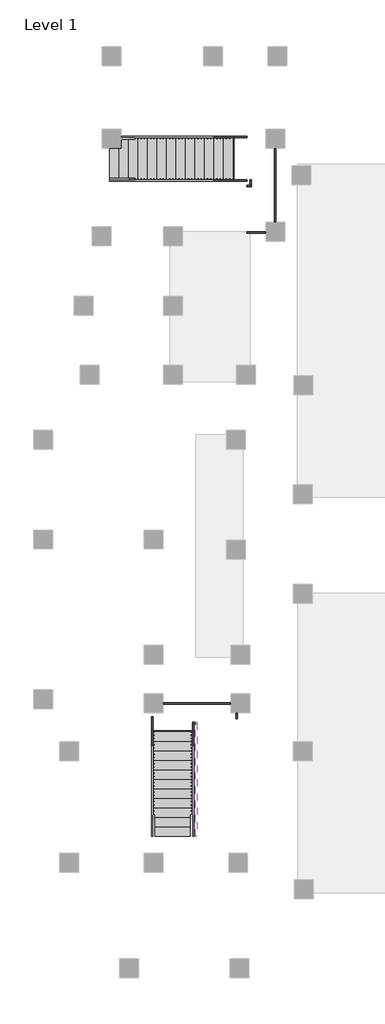
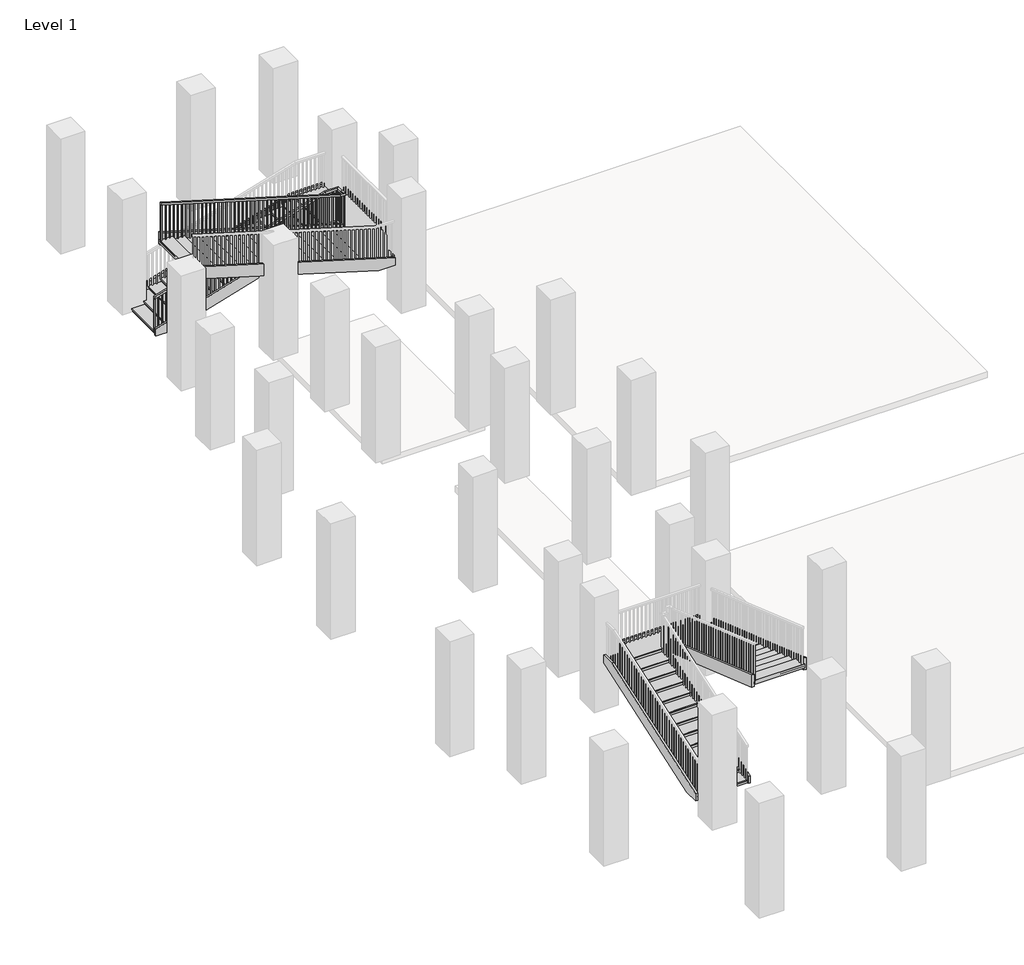
# One storey, part 6 of 6: 12 members, 2 stair flights, 1 railing.
"""IFC4 building model written with IfcOpenShell, lengths in millimetres."""

from ifc_helpers import new_model, si_unit, frame, origin, place, context, project, spatial, polyline, outline, extrude, faceted_brep, transform, mapped, element, save
from components import stair_flight_6e2526ab, stair_flight_f9fdc227

model = new_model("IFC4")

# Units and contexts
model_context = context("Model", 3, world=origin())
ifc_project = project(units=[si_unit("LENGTHUNIT", "METRE", prefix="MILLI")], contexts=[model_context])

# Site, building, storey
site = spatial("IfcSite", under=ifc_project)
building = spatial("IfcBuilding", under=site)
storey = spatial("IfcBuildingStorey", under=building, Name="Level 1", Elevation=0.0)

# Members
placement = place(None, origin())
element("IfcMember", 1, ObjectType="Stringer - 2\" Width", at=placement, inside=storey, context=model_context, shape_type="SweptSolid", body=[
    extrude(outline(polyline([(-9955.5916506, 0.0), (-9955.5916506, 191.3592169), (-6325.8738327, 1447.8), (-5713.7916506, 1447.8), (-5713.7916506, 1337.1301656), (-9576.612129, 0.0), (-9955.5916506, 0.0)])), frame((-3908.487215, 0.0, 0.0), z_axis=(1.0, 0.0, 0.0), x_axis=(0.0, 1.0, 0.0)), (0.0, 0.0, 1.0), 50.8),
])
element("IfcMember", 2, ObjectType="Stringer - 2\" Width", at=placement, inside=storey, context=model_context, shape_type="SweptSolid", body=[
    extrude(outline(polyline([(-3908.487215, -5713.7916506), (-3908.487215, -5662.9916506), (-1190.687215, -5662.9916506), (-1190.687215, -5713.7916506), (-3908.487215, -5713.7916506)])), frame((0.0, 0.0, 1143.0), z_axis=(0.0, 0.0, 1.0), x_axis=(1.0, 0.0, 0.0)), (0.0, 0.0, 1.0), 304.8),
])
element("IfcMember", 3, ObjectType="Stringer - 2\" Width", at=placement, inside=storey, context=model_context, shape_type="SweptSolid", body=[
    extrude(outline(polyline([(-5662.9916506, 1347.5476784), (-5662.9916506, 1143.0), (-6003.8711722, 1143.0), (-9949.2416506, 2508.7051656), (-9949.2416506, 2831.2496015), (-5662.9916506, 1347.5476784)])), frame((-1190.687215, 0.0, 0.0), z_axis=(1.0, 0.0, 0.0), x_axis=(0.0, 1.0, 0.0)), (0.0, 0.0, 1.0), 50.8),
])
element("IfcMember", 4, ObjectType="Stringer - 2\" Width", at=placement, inside=storey, context=model_context, shape_type="SweptSolid", body=[
    extrude(outline(polyline([(-9955.5916506, 0.0), (-9955.5916506, 191.3592169), (-6342.4416506, 1442.0649861), (-6342.4416506, 1119.5205502), (-9576.612129, 0.0), (-9955.5916506, 0.0)])), frame((-2593.7381751, 0.0, 0.0), z_axis=(1.0, 0.0, 0.0), x_axis=(0.0, 1.0, 0.0)), (0.0, 0.0, 1.0), 50.8),
])
element("IfcMember", 5, ObjectType="Stringer - 2\" Width", at=placement, inside=storey, context=model_context, shape_type="SweptSolid", body=[
    extrude(outline(polyline([(-2593.7381751, -6342.4416506), (-2593.7381751, -6291.6416506), (-2492.1381751, -6291.6416506), (-2492.1381751, -6342.4416506), (-2593.7381751, -6342.4416506)])), frame((0.0, 0.0, 1143.0), z_axis=(0.0, 0.0, 1.0), x_axis=(1.0, 0.0, 0.0)), (0.0, 0.0, 1.0), 304.8),
])
element("IfcMember", 6, ObjectType="Stringer - 2\" Width", at=placement, inside=storey, context=model_context, shape_type="SweptSolid", body=[
    extrude(outline(polyline([(-6291.6416506, 1565.1572938), (-6291.6416506, 1242.6128579), (-9949.2416506, 2508.7051656), (-9949.2416506, 2831.2496015), (-6291.6416506, 1565.1572938)])), frame((-2492.1381751, 0.0, 0.0), z_axis=(1.0, 0.0, 0.0), x_axis=(0.0, 1.0, 0.0)), (0.0, 0.0, 1.0), 50.8),
])
element("IfcMember", 7, ObjectType="Stringer - 2\" Width", at=placement, inside=storey, context=model_context, shape_type="SweptSolid", body=[
    extrude(outline(polyline([(191.5995961, -5254.0891351), (0.0, -5254.0891351), (0.0, -4832.019314), (1447.8, -6.019314), (1447.8, -1066.7544553), (191.5995961, -5254.0891351)])), frame((0.0, 12506.0715905, 0.0), z_axis=(0.0, 1.0, 0.0), x_axis=(0.0, 0.0, 1.0)), (0.0, 0.0, 1.0), 50.8),
])
element("IfcMember", 8, ObjectType="Stringer - 2\" Width", at=placement, inside=storey, context=model_context, shape_type="SweptSolid", body=[
    extrude(outline(polyline([(54.5108649, 12556.8715905), (105.3108649, 12556.8715905), (105.3108649, 9478.4949943), (54.5108649, 9478.4949943), (54.5108649, 12556.8715905)])), frame((0.0, 0.0, 1143.0), z_axis=(0.0, 0.0, 1.0), x_axis=(1.0, 0.0, 0.0)), (0.0, 0.0, 1.0), 304.8),
])
element("IfcMember", 9, ObjectType="Stringer - 2\" Width", at=placement, inside=storey, context=model_context, shape_type="SweptSolid", body=[
    extrude(outline(polyline([(1143.0, 105.3108649), (1235.5395961, 105.3108649), (2843.3595961, -5254.0891351), (2525.1390537, -5254.0891351), (1143.0, -646.9589562), (1143.0, 105.3108649)])), frame((0.0, 9427.6949943, 0.0), z_axis=(0.0, 1.0, 0.0), x_axis=(0.0, 0.0, 1.0)), (0.0, 0.0, 1.0), 50.8),
])
element("IfcMember", 10, ObjectType="Stringer - 2\" Width", at=placement, inside=storey, context=model_context, shape_type="SweptSolid", body=[
    extrude(outline(polyline([(191.5995961, -5254.0891351), (0.0, -5254.0891351), (0.0, -4832.019314), (1229.7390537, -732.8891351), (1447.8, -732.8891351), (1447.8, -1066.7544553), (191.5995961, -5254.0891351)])), frame((0.0, 11103.4082924, 0.0), z_axis=(0.0, 1.0, 0.0), x_axis=(0.0, 0.0, 1.0)), (0.0, 0.0, 1.0), 50.8),
])
element("IfcMember", 11, ObjectType="Stringer - 2\" Width", at=placement, inside=storey, context=model_context, shape_type="SweptSolid", body=[
    extrude(outline(polyline([(-732.8891351, 11154.2082924), (-682.0891351, 11154.2082924), (-682.0891351, 10976.4082924), (-732.8891351, 10976.4082924), (-732.8891351, 11154.2082924)])), frame((0.0, 0.0, 1143.0), z_axis=(0.0, 0.0, 1.0), x_axis=(1.0, 0.0, 0.0)), (0.0, 0.0, 1.0), 304.8),
])
element("IfcMember", 12, ObjectType="Stringer - 2\" Width", at=placement, inside=storey, context=model_context, shape_type="SweptSolid", body=[
    extrude(outline(polyline([(1153.5390537, -682.0891351), (1471.7595961, -682.0891351), (2843.3595961, -5254.0891351), (2525.1390537, -5254.0891351), (1153.5390537, -682.0891351)])), frame((0.0, 10925.6082924, 0.0), z_axis=(0.0, 1.0, 0.0), x_axis=(0.0, 0.0, 1.0)), (0.0, 0.0, 1.0), 50.8),
])

# Railing
element("IfcRailing", 13, ObjectType="Handrail - Rectangular", at=placement, inside=storey, context=model_context, shape_type="SolidModel", body=[
    faceted_brep([(-5254.0891351, 11205.0082924, 1005.84), (-5254.0891351, 11205.0082924, 952.8032429), (-5254.0891351, 11154.2082924, 952.8032429), (-5254.0891351, 11154.2082924, 1005.84), (-986.8891351, 11205.0082924, 2286.0), (-979.4332782, 11205.0082924, 2235.2), (-979.4332782, 11154.2082924, 2235.2), (-986.8891351, 11154.2082924, 2286.0), (-631.2891351, 11205.0082924, 2286.0), (-631.2891351, 11205.0082924, 2235.2), (-682.0891351, 11154.2082924, 2235.2), (-682.0891351, 11154.2082924, 2286.0), (-631.2891351, 11001.8082924, 2286.0), (-631.2891351, 10951.0082924, 2235.2), (-682.0891351, 10951.0082924, 2235.2), (-682.0891351, 11001.8082924, 2286.0), (-631.2891351, 11001.8082924, 2308.86), (-631.2891351, 10951.0082924, 2258.06), (-682.0891351, 10951.0082924, 2258.06), (-682.0891351, 11001.8082924, 2308.86), (-631.2891351, 10874.8082924, 2308.86), (-631.2891351, 10874.8082924, 2258.06), (-682.0891351, 10925.6082924, 2258.06), (-682.0891351, 10925.6082924, 2308.86), (-758.2891351, 10874.8082924, 2308.86), (-765.744992, 10874.8082924, 2258.06), (-765.744992, 10925.6082924, 2258.06), (-758.2891351, 10925.6082924, 2308.86), (-5254.0891351, 10874.8082924, 3657.6), (-5254.0891351, 10925.6082924, 3657.6), (-5254.0891351, 10925.6082924, 3604.5632429), (-5254.0891351, 10874.8082924, 3604.5632429)], [[[0, 1, 2, 3]], [[1, 0, 4, 5]], [[2, 1, 5, 6]], [[3, 2, 6, 7]], [[0, 3, 7, 4]], [[5, 4, 8, 9]], [[6, 5, 9, 10]], [[7, 6, 10, 11]], [[4, 7, 11, 8]], [[9, 8, 12, 13]], [[10, 9, 13, 14]], [[11, 10, 14, 15]], [[8, 11, 15, 12]], [[13, 12, 16, 17]], [[14, 13, 17, 18]], [[15, 14, 18, 19]], [[12, 15, 19, 16]], [[17, 16, 20, 21]], [[18, 17, 21, 22]], [[19, 18, 22, 23]], [[16, 19, 23, 20]], [[21, 20, 24, 25]], [[22, 21, 25, 26]], [[23, 22, 26, 27]], [[20, 23, 27, 24]], [[28, 29, 30, 31]], [[25, 24, 28, 31]], [[26, 25, 31, 30]], [[27, 26, 30, 29]], [[24, 27, 29, 28]]]),
    extrude(outline(polyline([(3594.0857429, -5219.1641351), (3599.8007429, -5238.2141351), (2651.76, -5238.2141351), (2651.76, -5219.1641351), (3594.0857429, -5219.1641351)])), frame((0.0, 10890.6832924, 0.0), z_axis=(0.0, 1.0, 0.0), x_axis=(0.0, 0.0, 1.0)), (0.0, 0.0, 1.0), 19.05),
    extrude(outline(polyline([(3563.6057429, -5117.5641351), (3569.3207429, -5136.6141351), (2651.76, -5136.6141351), (2651.76, -5117.5641351), (3563.6057429, -5117.5641351)])), frame((0.0, 10890.6832924, 0.0), z_axis=(0.0, 1.0, 0.0), x_axis=(0.0, 0.0, 1.0)), (0.0, 0.0, 1.0), 19.05),
    extrude(outline(polyline([(3533.1257429, -5015.9641351), (3538.8407429, -5035.0141351), (2651.76, -5035.0141351), (2651.76, -5015.9641351), (3533.1257429, -5015.9641351)])), frame((0.0, 10890.6832924, 0.0), z_axis=(0.0, 1.0, 0.0), x_axis=(0.0, 0.0, 1.0)), (0.0, 0.0, 1.0), 19.05),
    extrude(outline(polyline([(3502.6457429, -4914.3641351), (3508.3607429, -4933.4141351), (2560.32, -4933.4141351), (2560.32, -4914.3641351), (3502.6457429, -4914.3641351)])), frame((0.0, 10890.6832924, 0.0), z_axis=(0.0, 1.0, 0.0), x_axis=(0.0, 0.0, 1.0)), (0.0, 0.0, 1.0), 19.05),
    extrude(outline(polyline([(3472.1657429, -4812.7641351), (3477.8807429, -4831.8141351), (2560.32, -4831.8141351), (2560.32, -4812.7641351), (3472.1657429, -4812.7641351)])), frame((0.0, 10890.6832924, 0.0), z_axis=(0.0, 1.0, 0.0), x_axis=(0.0, 0.0, 1.0)), (0.0, 0.0, 1.0), 19.05),
    extrude(outline(polyline([(3441.6857429, -4711.1641351), (3447.4007429, -4730.2141351), (2560.32, -4730.2141351), (2560.32, -4711.1641351), (3441.6857429, -4711.1641351)])), frame((0.0, 10890.6832924, 0.0), z_axis=(0.0, 1.0, 0.0), x_axis=(0.0, 0.0, 1.0)), (0.0, 0.0, 1.0), 19.05),
    extrude(outline(polyline([(3411.2057429, -4609.5641351), (3416.9207429, -4628.6141351), (2468.88, -4628.6141351), (2468.88, -4609.5641351), (3411.2057429, -4609.5641351)])), frame((0.0, 10890.6832924, 0.0), z_axis=(0.0, 1.0, 0.0), x_axis=(0.0, 0.0, 1.0)), (0.0, 0.0, 1.0), 19.05),
    extrude(outline(polyline([(3380.7257429, -4507.9641351), (3386.4407429, -4527.0141351), (2468.88, -4527.0141351), (2468.88, -4507.9641351), (3380.7257429, -4507.9641351)])), frame((0.0, 10890.6832924, 0.0), z_axis=(0.0, 1.0, 0.0), x_axis=(0.0, 0.0, 1.0)), (0.0, 0.0, 1.0), 19.05),
    extrude(outline(polyline([(3350.2457429, -4406.3641351), (3355.9607429, -4425.4141351), (2468.88, -4425.4141351), (2468.88, -4406.3641351), (3350.2457429, -4406.3641351)])), frame((0.0, 10890.6832924, 0.0), z_axis=(0.0, 1.0, 0.0), x_axis=(0.0, 0.0, 1.0)), (0.0, 0.0, 1.0), 19.05),
    extrude(outline(polyline([(3319.7657429, -4304.7641351), (3325.4807429, -4323.8141351), (2377.44, -4323.8141351), (2377.44, -4304.7641351), (3319.7657429, -4304.7641351)])), frame((0.0, 10890.6832924, 0.0), z_axis=(0.0, 1.0, 0.0), x_axis=(0.0, 0.0, 1.0)), (0.0, 0.0, 1.0), 19.05),
    extrude(outline(polyline([(3289.2857429, -4203.1641351), (3295.0007429, -4222.2141351), (2377.44, -4222.2141351), (2377.44, -4203.1641351), (3289.2857429, -4203.1641351)])), frame((0.0, 10890.6832924, 0.0), z_axis=(0.0, 1.0, 0.0), x_axis=(0.0, 0.0, 1.0)), (0.0, 0.0, 1.0), 19.05),
    extrude(outline(polyline([(3258.8057429, -4101.5641351), (3264.5207429, -4120.6141351), (2377.44, -4120.6141351), (2377.44, -4101.5641351), (3258.8057429, -4101.5641351)])), frame((0.0, 10890.6832924, 0.0), z_axis=(0.0, 1.0, 0.0), x_axis=(0.0, 0.0, 1.0)), (0.0, 0.0, 1.0), 19.05),
    extrude(outline(polyline([(3228.3257429, -3999.9641351), (3234.0407429, -4019.0141351), (2286.0, -4019.0141351), (2286.0, -3999.9641351), (3228.3257429, -3999.9641351)])), frame((0.0, 10890.6832924, 0.0), z_axis=(0.0, 1.0, 0.0), x_axis=(0.0, 0.0, 1.0)), (0.0, 0.0, 1.0), 19.05),
    extrude(outline(polyline([(3197.8457429, -3898.3641351), (3203.5607429, -3917.4141351), (2286.0, -3917.4141351), (2286.0, -3898.3641351), (3197.8457429, -3898.3641351)])), frame((0.0, 10890.6832924, 0.0), z_axis=(0.0, 1.0, 0.0), x_axis=(0.0, 0.0, 1.0)), (0.0, 0.0, 1.0), 19.05),
    extrude(outline(polyline([(3167.3657429, -3796.7641351), (3173.0807429, -3815.8141351), (2286.0, -3815.8141351), (2286.0, -3796.7641351), (3167.3657429, -3796.7641351)])), frame((0.0, 10890.6832924, 0.0), z_axis=(0.0, 1.0, 0.0), x_axis=(0.0, 0.0, 1.0)), (0.0, 0.0, 1.0), 19.05),
    extrude(outline(polyline([(3136.8857429, -3695.1641351), (3142.6007429, -3714.2141351), (2194.56, -3714.2141351), (2194.56, -3695.1641351), (3136.8857429, -3695.1641351)])), frame((0.0, 10890.6832924, 0.0), z_axis=(0.0, 1.0, 0.0), x_axis=(0.0, 0.0, 1.0)), (0.0, 0.0, 1.0), 19.05),
    extrude(outline(polyline([(3106.4057429, -3593.5641351), (3112.1207429, -3612.6141351), (2194.56, -3612.6141351), (2194.56, -3593.5641351), (3106.4057429, -3593.5641351)])), frame((0.0, 10890.6832924, 0.0), z_axis=(0.0, 1.0, 0.0), x_axis=(0.0, 0.0, 1.0)), (0.0, 0.0, 1.0), 19.05),
    extrude(outline(polyline([(3075.9257429, -3491.9641351), (3081.6407429, -3511.0141351), (2194.56, -3511.0141351), (2194.56, -3491.9641351), (3075.9257429, -3491.9641351)])), frame((0.0, 10890.6832924, 0.0), z_axis=(0.0, 1.0, 0.0), x_axis=(0.0, 0.0, 1.0)), (0.0, 0.0, 1.0), 19.05),
    extrude(outline(polyline([(3045.4457429, -3390.3641351), (3051.1607429, -3409.4141351), (2103.12, -3409.4141351), (2103.12, -3390.3641351), (3045.4457429, -3390.3641351)])), frame((0.0, 10890.6832924, 0.0), z_axis=(0.0, 1.0, 0.0), x_axis=(0.0, 0.0, 1.0)), (0.0, 0.0, 1.0), 19.05),
    extrude(outline(polyline([(3014.9657429, -3288.7641351), (3020.6807429, -3307.8141351), (2103.12, -3307.8141351), (2103.12, -3288.7641351), (3014.9657429, -3288.7641351)])), frame((0.0, 10890.6832924, 0.0), z_axis=(0.0, 1.0, 0.0), x_axis=(0.0, 0.0, 1.0)), (0.0, 0.0, 1.0), 19.05),
    extrude(outline(polyline([(2984.4857429, -3187.1641351), (2990.2007429, -3206.2141351), (2103.12, -3206.2141351), (2103.12, -3187.1641351), (2984.4857429, -3187.1641351)])), frame((0.0, 10890.6832924, 0.0), z_axis=(0.0, 1.0, 0.0), x_axis=(0.0, 0.0, 1.0)), (0.0, 0.0, 1.0), 19.05),
    extrude(outline(polyline([(2954.0057429, -3085.5641351), (2959.7207429, -3104.6141351), (2011.68, -3104.6141351), (2011.68, -3085.5641351), (2954.0057429, -3085.5641351)])), frame((0.0, 10890.6832924, 0.0), z_axis=(0.0, 1.0, 0.0), x_axis=(0.0, 0.0, 1.0)), (0.0, 0.0, 1.0), 19.05),
    extrude(outline(polyline([(2923.5257429, -2983.9641351), (2929.2407429, -3003.0141351), (2011.68, -3003.0141351), (2011.68, -2983.9641351), (2923.5257429, -2983.9641351)])), frame((0.0, 10890.6832924, 0.0), z_axis=(0.0, 1.0, 0.0), x_axis=(0.0, 0.0, 1.0)), (0.0, 0.0, 1.0), 19.05),
    extrude(outline(polyline([(2893.0457429, -2882.3641351), (2898.7607429, -2901.4141351), (2011.68, -2901.4141351), (2011.68, -2882.3641351), (2893.0457429, -2882.3641351)])), frame((0.0, 10890.6832924, 0.0), z_axis=(0.0, 1.0, 0.0), x_axis=(0.0, 0.0, 1.0)), (0.0, 0.0, 1.0), 19.05),
    extrude(outline(polyline([(2862.5657429, -2780.7641351), (2868.2807429, -2799.8141351), (1920.24, -2799.8141351), (1920.24, -2780.7641351), (2862.5657429, -2780.7641351)])), frame((0.0, 10890.6832924, 0.0), z_axis=(0.0, 1.0, 0.0), x_axis=(0.0, 0.0, 1.0)), (0.0, 0.0, 1.0), 19.05),
    extrude(outline(polyline([(2832.0857429, -2679.1641351), (2837.8007429, -2698.2141351), (1920.24, -2698.2141351), (1920.24, -2679.1641351), (2832.0857429, -2679.1641351)])), frame((0.0, 10890.6832924, 0.0), z_axis=(0.0, 1.0, 0.0), x_axis=(0.0, 0.0, 1.0)), (0.0, 0.0, 1.0), 19.05),
    extrude(outline(polyline([(2801.6057429, -2577.5641351), (2807.3207429, -2596.6141351), (1920.24, -2596.6141351), (1920.24, -2577.5641351), (2801.6057429, -2577.5641351)])), frame((0.0, 10890.6832924, 0.0), z_axis=(0.0, 1.0, 0.0), x_axis=(0.0, 0.0, 1.0)), (0.0, 0.0, 1.0), 19.05),
    extrude(outline(polyline([(2771.1257429, -2475.9641351), (2776.8407429, -2495.0141351), (1828.8, -2495.0141351), (1828.8, -2475.9641351), (2771.1257429, -2475.9641351)])), frame((0.0, 10890.6832924, 0.0), z_axis=(0.0, 1.0, 0.0), x_axis=(0.0, 0.0, 1.0)), (0.0, 0.0, 1.0), 19.05),
    extrude(outline(polyline([(2740.6457429, -2374.3641351), (2746.3607429, -2393.4141351), (1828.8, -2393.4141351), (1828.8, -2374.3641351), (2740.6457429, -2374.3641351)])), frame((0.0, 10890.6832924, 0.0), z_axis=(0.0, 1.0, 0.0), x_axis=(0.0, 0.0, 1.0)), (0.0, 0.0, 1.0), 19.05),
    extrude(outline(polyline([(2710.1657429, -2272.7641351), (2715.8807429, -2291.8141351), (1828.8, -2291.8141351), (1828.8, -2272.7641351), (2710.1657429, -2272.7641351)])), frame((0.0, 10890.6832924, 0.0), z_axis=(0.0, 1.0, 0.0), x_axis=(0.0, 0.0, 1.0)), (0.0, 0.0, 1.0), 19.05),
    extrude(outline(polyline([(2679.6857429, -2171.1641351), (2685.4007429, -2190.2141351), (1737.36, -2190.2141351), (1737.36, -2171.1641351), (2679.6857429, -2171.1641351)])), frame((0.0, 10890.6832924, 0.0), z_axis=(0.0, 1.0, 0.0), x_axis=(0.0, 0.0, 1.0)), (0.0, 0.0, 1.0), 19.05),
    extrude(outline(polyline([(2649.2057429, -2069.5641351), (2654.9207429, -2088.6141351), (1737.36, -2088.6141351), (1737.36, -2069.5641351), (2649.2057429, -2069.5641351)])), frame((0.0, 10890.6832924, 0.0), z_axis=(0.0, 1.0, 0.0), x_axis=(0.0, 0.0, 1.0)), (0.0, 0.0, 1.0), 19.05),
    extrude(outline(polyline([(2618.7257429, -1967.9641351), (2624.4407429, -1987.0141351), (1737.36, -1987.0141351), (1737.36, -1967.9641351), (2618.7257429, -1967.9641351)])), frame((0.0, 10890.6832924, 0.0), z_axis=(0.0, 1.0, 0.0), x_axis=(0.0, 0.0, 1.0)), (0.0, 0.0, 1.0), 19.05),
    extrude(outline(polyline([(2588.2457429, -1866.3641351), (2593.9607429, -1885.4141351), (1645.92, -1885.4141351), (1645.92, -1866.3641351), (2588.2457429, -1866.3641351)])), frame((0.0, 10890.6832924, 0.0), z_axis=(0.0, 1.0, 0.0), x_axis=(0.0, 0.0, 1.0)), (0.0, 0.0, 1.0), 19.05),
    extrude(outline(polyline([(2557.7657429, -1764.7641351), (2563.4807429, -1783.8141351), (1645.92, -1783.8141351), (1645.92, -1764.7641351), (2557.7657429, -1764.7641351)])), frame((0.0, 10890.6832924, 0.0), z_axis=(0.0, 1.0, 0.0), x_axis=(0.0, 0.0, 1.0)), (0.0, 0.0, 1.0), 19.05),
    extrude(outline(polyline([(2527.2857429, -1663.1641351), (2533.0007429, -1682.2141351), (1645.92, -1682.2141351), (1645.92, -1663.1641351), (2527.2857429, -1663.1641351)])), frame((0.0, 10890.6832924, 0.0), z_axis=(0.0, 1.0, 0.0), x_axis=(0.0, 0.0, 1.0)), (0.0, 0.0, 1.0), 19.05),
    extrude(outline(polyline([(2496.8057429, -1561.5641351), (2502.5207429, -1580.6141351), (1554.48, -1580.6141351), (1554.48, -1561.5641351), (2496.8057429, -1561.5641351)])), frame((0.0, 10890.6832924, 0.0), z_axis=(0.0, 1.0, 0.0), x_axis=(0.0, 0.0, 1.0)), (0.0, 0.0, 1.0), 19.05),
    extrude(outline(polyline([(2466.3257429, -1459.9641351), (2472.0407429, -1479.0141351), (1554.48, -1479.0141351), (1554.48, -1459.9641351), (2466.3257429, -1459.9641351)])), frame((0.0, 10890.6832924, 0.0), z_axis=(0.0, 1.0, 0.0), x_axis=(0.0, 0.0, 1.0)), (0.0, 0.0, 1.0), 19.05),
    extrude(outline(polyline([(2435.8457429, -1358.3641351), (2441.5607429, -1377.4141351), (1554.48, -1377.4141351), (1554.48, -1358.3641351), (2435.8457429, -1358.3641351)])), frame((0.0, 10890.6832924, 0.0), z_axis=(0.0, 1.0, 0.0), x_axis=(0.0, 0.0, 1.0)), (0.0, 0.0, 1.0), 19.05),
    extrude(outline(polyline([(2405.3657429, -1256.7641351), (2411.0807429, -1275.8141351), (1463.04, -1275.8141351), (1463.04, -1256.7641351), (2405.3657429, -1256.7641351)])), frame((0.0, 10890.6832924, 0.0), z_axis=(0.0, 1.0, 0.0), x_axis=(0.0, 0.0, 1.0)), (0.0, 0.0, 1.0), 19.05),
    extrude(outline(polyline([(2374.8857429, -1155.1641351), (2380.6007429, -1174.2141351), (1463.04, -1174.2141351), (1463.04, -1155.1641351), (2374.8857429, -1155.1641351)])), frame((0.0, 10890.6832924, 0.0), z_axis=(0.0, 1.0, 0.0), x_axis=(0.0, 0.0, 1.0)), (0.0, 0.0, 1.0), 19.05),
    extrude(outline(polyline([(2344.4057429, -1053.5641351), (2350.1207429, -1072.6141351), (1463.04, -1072.6141351), (1463.04, -1053.5641351), (2344.4057429, -1053.5641351)])), frame((0.0, 10890.6832924, 0.0), z_axis=(0.0, 1.0, 0.0), x_axis=(0.0, 0.0, 1.0)), (0.0, 0.0, 1.0), 19.05),
    extrude(outline(polyline([(2313.9257429, -951.9641351), (2319.6407429, -971.0141351), (1371.6, -971.0141351), (1371.6, -951.9641351), (2313.9257429, -951.9641351)])), frame((0.0, 10890.6832924, 0.0), z_axis=(0.0, 1.0, 0.0), x_axis=(0.0, 0.0, 1.0)), (0.0, 0.0, 1.0), 19.05),
    extrude(outline(polyline([(2283.4457429, -850.3641351), (2289.1607429, -869.4141351), (1371.6, -869.4141351), (1371.6, -850.3641351), (2283.4457429, -850.3641351)])), frame((0.0, 10890.6832924, 0.0), z_axis=(0.0, 1.0, 0.0), x_axis=(0.0, 0.0, 1.0)), (0.0, 0.0, 1.0), 19.05),
    extrude(outline(polyline([(2252.9657429, -748.7641351), (2258.6807429, -767.8141351), (1371.6, -767.8141351), (1371.6, -748.7641351), (2252.9657429, -748.7641351)])), frame((0.0, 10890.6832924, 0.0), z_axis=(0.0, 1.0, 0.0), x_axis=(0.0, 0.0, 1.0)), (0.0, 0.0, 1.0), 19.05),
    extrude(outline(polyline([(-666.2141351, 10985.9332924), (-647.1641351, 10985.9332924), (-647.1641351, 10966.8832924), (-666.2141351, 10966.8832924), (-666.2141351, 10985.9332924)])), frame((0.0, 0.0, 1371.6), z_axis=(0.0, 0.0, 1.0), x_axis=(1.0, 0.0, 0.0)), (0.0, 0.0, 1.0), 886.46),
    extrude(outline(polyline([(-666.2141351, 11087.5332924), (-647.1641351, 11087.5332924), (-647.1641351, 11068.4832924), (-666.2141351, 11068.4832924), (-666.2141351, 11087.5332924)])), frame((0.0, 0.0, 1371.6), z_axis=(0.0, 0.0, 1.0), x_axis=(1.0, 0.0, 0.0)), (0.0, 0.0, 1.0), 863.6),
    extrude(outline(polyline([(-691.6141351, 11170.0832924), (-691.6141351, 11189.1332924), (-672.5641351, 11189.1332924), (-672.5641351, 11170.0832924), (-691.6141351, 11170.0832924)])), frame((0.0, 0.0, 1371.6), z_axis=(0.0, 0.0, 1.0), x_axis=(1.0, 0.0, 0.0)), (0.0, 0.0, 1.0), 863.6),
    extrude(outline(polyline([(-793.2141351, 11170.0832924), (-793.2141351, 11189.1332924), (-774.1641351, 11189.1332924), (-774.1641351, 11170.0832924), (-793.2141351, 11170.0832924)])), frame((0.0, 0.0, 1371.6), z_axis=(0.0, 0.0, 1.0), x_axis=(1.0, 0.0, 0.0)), (0.0, 0.0, 1.0), 863.6),
    extrude(outline(polyline([(-894.8141351, 11170.0832924), (-894.8141351, 11189.1332924), (-875.7641351, 11189.1332924), (-875.7641351, 11170.0832924), (-894.8141351, 11170.0832924)])), frame((0.0, 0.0, 1371.6), z_axis=(0.0, 0.0, 1.0), x_axis=(1.0, 0.0, 0.0)), (0.0, 0.0, 1.0), 863.6),
    extrude(outline(polyline([(2235.8207429, -977.3641351), (2230.1057429, -996.4141351), (1371.6, -996.4141351), (1371.6, -977.3641351), (2235.8207429, -977.3641351)])), frame((0.0, 11170.0832924, 0.0), z_axis=(0.0, 1.0, 0.0), x_axis=(0.0, 0.0, 1.0)), (0.0, 0.0, 1.0), 19.05),
    extrude(outline(polyline([(2205.3407429, -1078.9641351), (2199.6257429, -1098.0141351), (1280.16, -1098.0141351), (1280.16, -1078.9641351), (2205.3407429, -1078.9641351)])), frame((0.0, 11170.0832924, 0.0), z_axis=(0.0, 1.0, 0.0), x_axis=(0.0, 0.0, 1.0)), (0.0, 0.0, 1.0), 19.05),
    extrude(outline(polyline([(2174.8607429, -1180.5641351), (2169.1457429, -1199.6141351), (1280.16, -1199.6141351), (1280.16, -1180.5641351), (2174.8607429, -1180.5641351)])), frame((0.0, 11170.0832924, 0.0), z_axis=(0.0, 1.0, 0.0), x_axis=(0.0, 0.0, 1.0)), (0.0, 0.0, 1.0), 19.05),
    extrude(outline(polyline([(2144.3807429, -1282.1641351), (2138.6657429, -1301.2141351), (1280.16, -1301.2141351), (1280.16, -1282.1641351), (2144.3807429, -1282.1641351)])), frame((0.0, 11170.0832924, 0.0), z_axis=(0.0, 1.0, 0.0), x_axis=(0.0, 0.0, 1.0)), (0.0, 0.0, 1.0), 19.05),
    extrude(outline(polyline([(2113.9007429, -1383.7641351), (2108.1857429, -1402.8141351), (1188.72, -1402.8141351), (1188.72, -1383.7641351), (2113.9007429, -1383.7641351)])), frame((0.0, 11170.0832924, 0.0), z_axis=(0.0, 1.0, 0.0), x_axis=(0.0, 0.0, 1.0)), (0.0, 0.0, 1.0), 19.05),
    extrude(outline(polyline([(2083.4207429, -1485.3641351), (2077.7057429, -1504.4141351), (1188.72, -1504.4141351), (1188.72, -1485.3641351), (2083.4207429, -1485.3641351)])), frame((0.0, 11170.0832924, 0.0), z_axis=(0.0, 1.0, 0.0), x_axis=(0.0, 0.0, 1.0)), (0.0, 0.0, 1.0), 19.05),
    extrude(outline(polyline([(2052.9407429, -1586.9641351), (2047.2257429, -1606.0141351), (1188.72, -1606.0141351), (1188.72, -1586.9641351), (2052.9407429, -1586.9641351)])), frame((0.0, 11170.0832924, 0.0), z_axis=(0.0, 1.0, 0.0), x_axis=(0.0, 0.0, 1.0)), (0.0, 0.0, 1.0), 19.05),
    extrude(outline(polyline([(2022.4607429, -1688.5641351), (2016.7457429, -1707.6141351), (1097.28, -1707.6141351), (1097.28, -1688.5641351), (2022.4607429, -1688.5641351)])), frame((0.0, 11170.0832924, 0.0), z_axis=(0.0, 1.0, 0.0), x_axis=(0.0, 0.0, 1.0)), (0.0, 0.0, 1.0), 19.05),
    extrude(outline(polyline([(1991.9807429, -1790.1641351), (1986.2657429, -1809.2141351), (1097.28, -1809.2141351), (1097.28, -1790.1641351), (1991.9807429, -1790.1641351)])), frame((0.0, 11170.0832924, 0.0), z_axis=(0.0, 1.0, 0.0), x_axis=(0.0, 0.0, 1.0)), (0.0, 0.0, 1.0), 19.05),
    extrude(outline(polyline([(1961.5007429, -1891.7641351), (1955.7857429, -1910.8141351), (1097.28, -1910.8141351), (1097.28, -1891.7641351), (1961.5007429, -1891.7641351)])), frame((0.0, 11170.0832924, 0.0), z_axis=(0.0, 1.0, 0.0), x_axis=(0.0, 0.0, 1.0)), (0.0, 0.0, 1.0), 19.05),
    extrude(outline(polyline([(1931.0207429, -1993.3641351), (1925.3057429, -2012.4141351), (1005.84, -2012.4141351), (1005.84, -1993.3641351), (1931.0207429, -1993.3641351)])), frame((0.0, 11170.0832924, 0.0), z_axis=(0.0, 1.0, 0.0), x_axis=(0.0, 0.0, 1.0)), (0.0, 0.0, 1.0), 19.05),
    extrude(outline(polyline([(1900.5407429, -2094.9641351), (1894.8257429, -2114.0141351), (1005.84, -2114.0141351), (1005.84, -2094.9641351), (1900.5407429, -2094.9641351)])), frame((0.0, 11170.0832924, 0.0), z_axis=(0.0, 1.0, 0.0), x_axis=(0.0, 0.0, 1.0)), (0.0, 0.0, 1.0), 19.05),
    extrude(outline(polyline([(1870.0607429, -2196.5641351), (1864.3457429, -2215.6141351), (1005.84, -2215.6141351), (1005.84, -2196.5641351), (1870.0607429, -2196.5641351)])), frame((0.0, 11170.0832924, 0.0), z_axis=(0.0, 1.0, 0.0), x_axis=(0.0, 0.0, 1.0)), (0.0, 0.0, 1.0), 19.05),
    extrude(outline(polyline([(1839.5807429, -2298.1641351), (1833.8657429, -2317.2141351), (914.4, -2317.2141351), (914.4, -2298.1641351), (1839.5807429, -2298.1641351)])), frame((0.0, 11170.0832924, 0.0), z_axis=(0.0, 1.0, 0.0), x_axis=(0.0, 0.0, 1.0)), (0.0, 0.0, 1.0), 19.05),
    extrude(outline(polyline([(1809.1007429, -2399.7641351), (1803.3857429, -2418.8141351), (914.4, -2418.8141351), (914.4, -2399.7641351), (1809.1007429, -2399.7641351)])), frame((0.0, 11170.0832924, 0.0), z_axis=(0.0, 1.0, 0.0), x_axis=(0.0, 0.0, 1.0)), (0.0, 0.0, 1.0), 19.05),
    extrude(outline(polyline([(1778.6207429, -2501.3641351), (1772.9057429, -2520.4141351), (914.4, -2520.4141351), (914.4, -2501.3641351), (1778.6207429, -2501.3641351)])), frame((0.0, 11170.0832924, 0.0), z_axis=(0.0, 1.0, 0.0), x_axis=(0.0, 0.0, 1.0)), (0.0, 0.0, 1.0), 19.05),
    extrude(outline(polyline([(1748.1407429, -2602.9641351), (1742.4257429, -2622.0141351), (822.96, -2622.0141351), (822.96, -2602.9641351), (1748.1407429, -2602.9641351)])), frame((0.0, 11170.0832924, 0.0), z_axis=(0.0, 1.0, 0.0), x_axis=(0.0, 0.0, 1.0)), (0.0, 0.0, 1.0), 19.05),
    extrude(outline(polyline([(1717.6607429, -2704.5641351), (1711.9457429, -2723.6141351), (822.96, -2723.6141351), (822.96, -2704.5641351), (1717.6607429, -2704.5641351)])), frame((0.0, 11170.0832924, 0.0), z_axis=(0.0, 1.0, 0.0), x_axis=(0.0, 0.0, 1.0)), (0.0, 0.0, 1.0), 19.05),
    extrude(outline(polyline([(1687.1807429, -2806.1641351), (1681.4657429, -2825.2141351), (822.96, -2825.2141351), (822.96, -2806.1641351), (1687.1807429, -2806.1641351)])), frame((0.0, 11170.0832924, 0.0), z_axis=(0.0, 1.0, 0.0), x_axis=(0.0, 0.0, 1.0)), (0.0, 0.0, 1.0), 19.05),
    extrude(outline(polyline([(1656.7007429, -2907.7641351), (1650.9857429, -2926.8141351), (731.52, -2926.8141351), (731.52, -2907.7641351), (1656.7007429, -2907.7641351)])), frame((0.0, 11170.0832924, 0.0), z_axis=(0.0, 1.0, 0.0), x_axis=(0.0, 0.0, 1.0)), (0.0, 0.0, 1.0), 19.05),
    extrude(outline(polyline([(1626.2207429, -3009.3641351), (1620.5057429, -3028.4141351), (731.52, -3028.4141351), (731.52, -3009.3641351), (1626.2207429, -3009.3641351)])), frame((0.0, 11170.0832924, 0.0), z_axis=(0.0, 1.0, 0.0), x_axis=(0.0, 0.0, 1.0)), (0.0, 0.0, 1.0), 19.05),
    extrude(outline(polyline([(1595.7407429, -3110.9641351), (1590.0257429, -3130.0141351), (731.52, -3130.0141351), (731.52, -3110.9641351), (1595.7407429, -3110.9641351)])), frame((0.0, 11170.0832924, 0.0), z_axis=(0.0, 1.0, 0.0), x_axis=(0.0, 0.0, 1.0)), (0.0, 0.0, 1.0), 19.05),
    extrude(outline(polyline([(1565.2607429, -3212.5641351), (1559.5457429, -3231.6141351), (640.08, -3231.6141351), (640.08, -3212.5641351), (1565.2607429, -3212.5641351)])), frame((0.0, 11170.0832924, 0.0), z_axis=(0.0, 1.0, 0.0), x_axis=(0.0, 0.0, 1.0)), (0.0, 0.0, 1.0), 19.05),
    extrude(outline(polyline([(1534.7807429, -3314.1641351), (1529.0657429, -3333.2141351), (640.08, -3333.2141351), (640.08, -3314.1641351), (1534.7807429, -3314.1641351)])), frame((0.0, 11170.0832924, 0.0), z_axis=(0.0, 1.0, 0.0), x_axis=(0.0, 0.0, 1.0)), (0.0, 0.0, 1.0), 19.05),
    extrude(outline(polyline([(1504.3007429, -3415.7641351), (1498.5857429, -3434.8141351), (640.08, -3434.8141351), (640.08, -3415.7641351), (1504.3007429, -3415.7641351)])), frame((0.0, 11170.0832924, 0.0), z_axis=(0.0, 1.0, 0.0), x_axis=(0.0, 0.0, 1.0)), (0.0, 0.0, 1.0), 19.05),
    extrude(outline(polyline([(1473.8207429, -3517.3641351), (1468.1057429, -3536.4141351), (548.64, -3536.4141351), (548.64, -3517.3641351), (1473.8207429, -3517.3641351)])), frame((0.0, 11170.0832924, 0.0), z_axis=(0.0, 1.0, 0.0), x_axis=(0.0, 0.0, 1.0)), (0.0, 0.0, 1.0), 19.05),
    extrude(outline(polyline([(1443.3407429, -3618.9641351), (1437.6257429, -3638.0141351), (548.64, -3638.0141351), (548.64, -3618.9641351), (1443.3407429, -3618.9641351)])), frame((0.0, 11170.0832924, 0.0), z_axis=(0.0, 1.0, 0.0), x_axis=(0.0, 0.0, 1.0)), (0.0, 0.0, 1.0), 19.05),
    extrude(outline(polyline([(1412.8607429, -3720.5641351), (1407.1457429, -3739.6141351), (548.64, -3739.6141351), (548.64, -3720.5641351), (1412.8607429, -3720.5641351)])), frame((0.0, 11170.0832924, 0.0), z_axis=(0.0, 1.0, 0.0), x_axis=(0.0, 0.0, 1.0)), (0.0, 0.0, 1.0), 19.05),
    extrude(outline(polyline([(1382.3807429, -3822.1641351), (1376.6657429, -3841.2141351), (457.2, -3841.2141351), (457.2, -3822.1641351), (1382.3807429, -3822.1641351)])), frame((0.0, 11170.0832924, 0.0), z_axis=(0.0, 1.0, 0.0), x_axis=(0.0, 0.0, 1.0)), (0.0, 0.0, 1.0), 19.05),
    extrude(outline(polyline([(1351.9007429, -3923.7641351), (1346.1857429, -3942.8141351), (457.2, -3942.8141351), (457.2, -3923.7641351), (1351.9007429, -3923.7641351)])), frame((0.0, 11170.0832924, 0.0), z_axis=(0.0, 1.0, 0.0), x_axis=(0.0, 0.0, 1.0)), (0.0, 0.0, 1.0), 19.05),
    extrude(outline(polyline([(1321.4207429, -4025.3641351), (1315.7057429, -4044.4141351), (457.2, -4044.4141351), (457.2, -4025.3641351), (1321.4207429, -4025.3641351)])), frame((0.0, 11170.0832924, 0.0), z_axis=(0.0, 1.0, 0.0), x_axis=(0.0, 0.0, 1.0)), (0.0, 0.0, 1.0), 19.05),
    extrude(outline(polyline([(1290.9407429, -4126.9641351), (1285.2257429, -4146.0141351), (365.76, -4146.0141351), (365.76, -4126.9641351), (1290.9407429, -4126.9641351)])), frame((0.0, 11170.0832924, 0.0), z_axis=(0.0, 1.0, 0.0), x_axis=(0.0, 0.0, 1.0)), (0.0, 0.0, 1.0), 19.05),
    extrude(outline(polyline([(1260.4607429, -4228.5641351), (1254.7457429, -4247.6141351), (365.76, -4247.6141351), (365.76, -4228.5641351), (1260.4607429, -4228.5641351)])), frame((0.0, 11170.0832924, 0.0), z_axis=(0.0, 1.0, 0.0), x_axis=(0.0, 0.0, 1.0)), (0.0, 0.0, 1.0), 19.05),
    extrude(outline(polyline([(1229.9807429, -4330.1641351), (1224.2657429, -4349.2141351), (365.76, -4349.2141351), (365.76, -4330.1641351), (1229.9807429, -4330.1641351)])), frame((0.0, 11170.0832924, 0.0), z_axis=(0.0, 1.0, 0.0), x_axis=(0.0, 0.0, 1.0)), (0.0, 0.0, 1.0), 19.05),
    extrude(outline(polyline([(1199.5007429, -4431.7641351), (1193.7857429, -4450.8141351), (274.32, -4450.8141351), (274.32, -4431.7641351), (1199.5007429, -4431.7641351)])), frame((0.0, 11170.0832924, 0.0), z_axis=(0.0, 1.0, 0.0), x_axis=(0.0, 0.0, 1.0)), (0.0, 0.0, 1.0), 19.05),
    extrude(outline(polyline([(1169.0207429, -4533.3641351), (1163.3057429, -4552.4141351), (274.32, -4552.4141351), (274.32, -4533.3641351), (1169.0207429, -4533.3641351)])), frame((0.0, 11170.0832924, 0.0), z_axis=(0.0, 1.0, 0.0), x_axis=(0.0, 0.0, 1.0)), (0.0, 0.0, 1.0), 19.05),
    extrude(outline(polyline([(1138.5407429, -4634.9641351), (1132.8257429, -4654.0141351), (274.32, -4654.0141351), (274.32, -4634.9641351), (1138.5407429, -4634.9641351)])), frame((0.0, 11170.0832924, 0.0), z_axis=(0.0, 1.0, 0.0), x_axis=(0.0, 0.0, 1.0)), (0.0, 0.0, 1.0), 19.05),
    extrude(outline(polyline([(1108.0607429, -4736.5641351), (1102.3457429, -4755.6141351), (182.88, -4755.6141351), (182.88, -4736.5641351), (1108.0607429, -4736.5641351)])), frame((0.0, 11170.0832924, 0.0), z_axis=(0.0, 1.0, 0.0), x_axis=(0.0, 0.0, 1.0)), (0.0, 0.0, 1.0), 19.05),
    extrude(outline(polyline([(1077.5807429, -4838.1641351), (1071.8657429, -4857.2141351), (182.88, -4857.2141351), (182.88, -4838.1641351), (1077.5807429, -4838.1641351)])), frame((0.0, 11170.0832924, 0.0), z_axis=(0.0, 1.0, 0.0), x_axis=(0.0, 0.0, 1.0)), (0.0, 0.0, 1.0), 19.05),
    extrude(outline(polyline([(1047.1007429, -4939.7641351), (1041.3857429, -4958.8141351), (182.88, -4958.8141351), (182.88, -4939.7641351), (1047.1007429, -4939.7641351)])), frame((0.0, 11170.0832924, 0.0), z_axis=(0.0, 1.0, 0.0), x_axis=(0.0, 0.0, 1.0)), (0.0, 0.0, 1.0), 19.05),
    extrude(outline(polyline([(1016.6207429, -5041.3641351), (1010.9057429, -5060.4141351), (91.44, -5060.4141351), (91.44, -5041.3641351), (1016.6207429, -5041.3641351)])), frame((0.0, 11170.0832924, 0.0), z_axis=(0.0, 1.0, 0.0), x_axis=(0.0, 0.0, 1.0)), (0.0, 0.0, 1.0), 19.05),
    extrude(outline(polyline([(986.1407429, -5142.9641351), (980.4257429, -5162.0141351), (91.44, -5162.0141351), (91.44, -5142.9641351), (986.1407429, -5142.9641351)])), frame((0.0, 11170.0832924, 0.0), z_axis=(0.0, 1.0, 0.0), x_axis=(0.0, 0.0, 1.0)), (0.0, 0.0, 1.0), 19.05),
    extrude(outline(polyline([(-666.2141351, 10909.7332924), (-647.1641351, 10909.7332924), (-647.1641351, 10890.6832924), (-666.2141351, 10890.6832924), (-666.2141351, 10909.7332924)])), frame((0.0, 0.0, 1371.6), z_axis=(0.0, 0.0, 1.0), x_axis=(1.0, 0.0, 0.0)), (0.0, 0.0, 1.0), 886.46),
    extrude(outline(polyline([(-666.2141351, 11170.0832924), (-666.2141351, 11189.1332924), (-647.1641351, 11189.1332924), (-647.1641351, 11170.0832924), (-666.2141351, 11170.0832924)])), frame((0.0, 0.0, 1371.6), z_axis=(0.0, 0.0, 1.0), x_axis=(1.0, 0.0, 0.0)), (0.0, 0.0, 1.0), 863.6),
    extrude(outline(polyline([(3598.8482429, -5235.0391351), (3604.5632429, -5254.0891351), (2651.76, -5254.0891351), (2651.76, -5235.0391351), (3598.8482429, -5235.0391351)])), frame((0.0, 10890.6832924, 0.0), z_axis=(0.0, 1.0, 0.0), x_axis=(0.0, 0.0, 1.0)), (0.0, 0.0, 1.0), 19.05),
    extrude(outline(polyline([(958.5182429, -5235.0391351), (952.8032429, -5254.0891351), (91.44, -5254.0891351), (91.44, -5235.0391351), (958.5182429, -5235.0391351)])), frame((0.0, 11170.0832924, 0.0), z_axis=(0.0, 1.0, 0.0), x_axis=(0.0, 0.0, 1.0)), (0.0, 0.0, 1.0), 19.05),
])

# Stair flights
stair_flight_shape = stair_flight_6e2526ab(model_context)
element("IfcStairFlight", 14, ObjectType="2\" Tread 1\" Nosing 1/4\" Riser", at=placement, inside=storey, context=model_context, shape_type="MappedRepresentation", body=[
    mapped(stair_flight_shape, transform((0.0, 0.0, 0.0), x_axis=(1.0, 0.0, 0.0), y_axis=(0.0, 1.0, 0.0), z_axis=(0.0, 0.0, 1.0))),
])
stair_flight_2_shape = stair_flight_f9fdc227(model_context)
element("IfcStairFlight", 15, ObjectType="2\" Tread 1\" Nosing 1/4\" Riser", at=placement, inside=storey, context=model_context, shape_type="MappedRepresentation", body=[
    mapped(stair_flight_2_shape, transform((0.0, 0.0, 0.0), x_axis=(1.0, 0.0, 0.0), y_axis=(0.0, 1.0, 0.0), z_axis=(0.0, 0.0, 1.0))),
])

save(model, "model.ifc")

# Revit data of these elements
# Type "Handrail - Rectangular"
#   Assembly Code = "C2010400"
#   built-in parameter 1008612 = 0.0416667 (stored number, unit not read)
#   built-in parameter 1008611 = 0.0416667 (stored number, unit not read)
#   built-in parameter 1008609 = 0.333333 (stored number, unit not read)
#   built-in parameter 1008604 = 0.166667 (stored number, unit not read)
#   built-in parameter 1008603 = 0.166667 (stored number, unit not read)
#   Railing Height = 3' - 0"
#   built-in parameter 1008630 = 2
#   built-in parameter 1008610 = 2
#   built-in parameter 1008618 = Baluster - Square : 3/4"
# Elements 1, 2, 3, 5, 6, 7, 8, 9, 10, 11, 12 (IfcMember, "Stringer - 2\" Width")
#   Phase Created = New Construction
# Element 4 (IfcMember, "Stringer - 2\" Width")
#   Phase Created = New Construction
#   Materials on its faces: "Wood - Stained"
# Element 13 (IfcRailing, "Handrail - Rectangular")
#   Phase Created = New Construction
# Elements 14, 15 (IfcStairFlight, "2\" Tread 1\" Nosing 1/4\" Riser")
#   Phase Created = New Construction
# Materials
#   "Wood - Stained": class "Wood", colour RGB 224 178 126, transparency 0, Cost = 0
